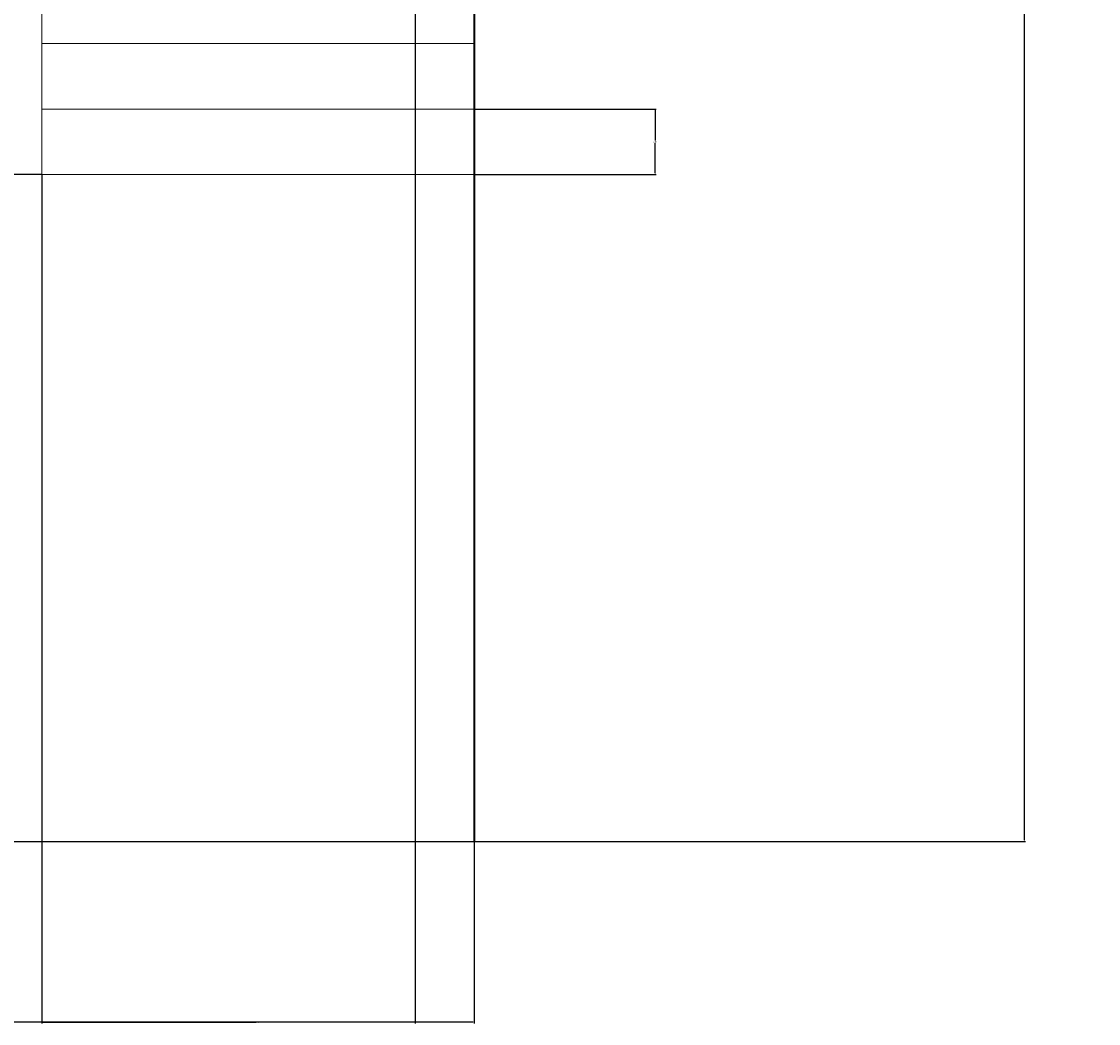
# Model space of a CAD drawing. Units: inches. Extents: x -4347 to -3836, y 955 to 1521.
# Tile 7 of 11: x -4001 to -3836, y 967 to 1120. Entities that reach past the tile are written whole.
import ezdxf

# ---------------------------------------------------------------- set-up
doc = ezdxf.new("R2010")
doc.units = ezdxf.units.IN
doc.header["$MEASUREMENT"] = 0
for name, color, linetype, lineweight in [('A-ANNO-DIMS', 2, 'Continuous', 18), ('A-FLOR', 7, 'Continuous', 25), ('A-FLOR-STRS', 7, 'Continuous', 18), ('A-WALL', 7, 'Continuous', 35)]:
    doc.layers.add(name, color=color, linetype=linetype, lineweight=lineweight)
doc.styles.get("Standard").update_dxf_attribs({"font": 'arial.ttf'})
doc.dimstyles.get("Standard").update_dxf_attribs({"dimtxt": 0.18, "dimasz": 0.18, "dimexe": 0.18, "dimexo": 0.0625, "dimgap": 0.09, "dimtad": 0, "dimtih": 1, "dimtoh": 1, "dimdec": 0, "dimzin": 0, "dimdsep": 46, "dimlunit": 3, "dimtxsty": 'Standard', "dimcen": 0.09, "dimadec": 0, "dimazin": 0, "dimtfac": 1, "dimtdec": 0, "dimtofl": 0, "dimtmove": 0, "dimatfit": 3, "dimfxl": 1, "dimtolj": 1, "dimtzin": 0, "dimarcsym": 0})

# ---------------------------------------------------------------- blocks, each defined once
blk = doc.blocks.new('*D2')
at = {"layer": 'A-ANNO-DIMS', "color": 0, "lineweight": -2, "transparency": 16777216}
for p, q in [((-3931.52, 1489.79), (-3847.29, 1489.79)), ((-3847.47, 1489.61), (-3847.47, 1245.44)), ((-3847.47, 994.97), (-3847.47, 1239.13)), ((-3931.52, 994.79), (-3847.29, 994.79))]:
    blk.add_line(p, q, dxfattribs=at)
at = {"layer": 'A-ANNO-DIMS', "color": 0, "transparency": 16777216}
for points in [[(-3847.5, 1489.61), (-3847.44, 1489.61), (-3847.47, 1489.79)], [(-3847.5, 994.97), (-3847.44, 994.97), (-3847.47, 994.79)]]:
    blk.add_solid(points, dxfattribs=at)
at = {"layer": 'Defpoints', "color": 0, "transparency": 16777216}
for p in [(-3931.58, 1489.79), (-3931.58, 994.79), (-3847.47, 994.79)]:
    blk.add_point(p, dxfattribs=at)
at = {"layer": 'A-ANNO-DIMS', "color": 0, "transparency": 16777216, "insert": (-3847.47, 1242.29), "char_height": 6, "attachment_point": 5}
blk.add_mtext('\\A1;41\'-3"', dxfattribs=at)
blk = doc.blocks.new('*D47')
at = {"layer": 'A-ANNO-DIMS', "color": 0, "lineweight": -2, "transparency": 16777216}
for p, q in [((-4120.58, 1288.73), (-4120.58, 966.96)), ((-3940.58, 1288.73), (-3940.58, 966.96)), ((-4120.4, 967.14), (-4030.97, 967.14)), ((-3940.76, 967.14), (-4030.19, 967.14))]:
    blk.add_line(p, q, dxfattribs=at)
at = {"layer": 'A-ANNO-DIMS', "color": 0, "transparency": 16777216}
for points in [[(-4120.4, 967.17), (-4120.4, 967.11), (-4120.58, 967.14)], [(-3940.76, 967.17), (-3940.76, 967.11), (-3940.58, 967.14)]]:
    blk.add_solid(points, dxfattribs=at)
at = {"layer": 'Defpoints', "color": 0, "transparency": 16777216}
for p in [(-4120.58, 1288.79), (-3940.58, 1288.79), (-3940.58, 967.14)]:
    blk.add_point(p, dxfattribs=at)
at = {"layer": 'A-ANNO-DIMS', "color": 0, "transparency": 16777216, "insert": (-4030.58, 967.14), "char_height": 0.18, "attachment_point": 5}
blk.add_mtext('\\A1;15\'-0"', dxfattribs=at)
blk = doc.blocks.new('*D52')
at = {"layer": 'A-ANNO-DIMS', "color": 0, "lineweight": -2, "transparency": 16777216}
for p, q in [((-3997.69, 1096.73), (-3997.69, 966.96)), ((-3931.58, 1096.73), (-3931.58, 966.96)), ((-3997.51, 967.14), (-3964.97, 967.14)), ((-3931.76, 967.14), (-3964.31, 967.14))]:
    blk.add_line(p, q, dxfattribs=at)
at = {"layer": 'A-ANNO-DIMS', "color": 0, "transparency": 16777216}
for points in [[(-3997.51, 967.17), (-3997.51, 967.11), (-3997.69, 967.14)], [(-3931.76, 967.17), (-3931.76, 967.11), (-3931.58, 967.14)]]:
    blk.add_solid(points, dxfattribs=at)
at = {"layer": 'Defpoints', "color": 0, "transparency": 16777216}
for p in [(-3997.69, 1096.79), (-3931.58, 1096.79), (-3931.58, 967.14)]:
    blk.add_point(p, dxfattribs=at)
at = {"layer": 'A-ANNO-DIMS', "color": 0, "transparency": 16777216, "insert": (-3964.64, 967.14), "char_height": 0.18, "attachment_point": 5}
blk.add_mtext('\\A1;5\'-6"', dxfattribs=at)
blk = doc.blocks.new('*D54')
at = {"layer": 'A-ANNO-DIMS', "color": 0, "lineweight": -2, "transparency": 16777216}
for p, q in [((-3997.76, 1126.79), (-4346.41, 1126.79)), ((-4346.23, 1126.61), (-4346.23, 1111.97)), ((-4346.23, 1096.97), (-4346.23, 1111.61)), ((-3997.76, 1096.79), (-4346.41, 1096.79))]:
    blk.add_line(p, q, dxfattribs=at)
at = {"layer": 'A-ANNO-DIMS', "color": 0, "transparency": 16777216}
for points in [[(-4346.26, 1126.61), (-4346.2, 1126.61), (-4346.23, 1126.79)], [(-4346.26, 1096.97), (-4346.2, 1096.97), (-4346.23, 1096.79)]]:
    blk.add_solid(points, dxfattribs=at)
at = {"layer": 'Defpoints', "color": 0, "transparency": 16777216}
for p in [(-4346.23, 1126.79), (-3997.69, 1126.79), (-3997.69, 1096.79)]:
    blk.add_point(p, dxfattribs=at)
at = {"layer": 'A-ANNO-DIMS', "color": 0, "transparency": 16777216, "insert": (-4346.23, 1111.79), "char_height": 0.18, "attachment_point": 5}
blk.add_mtext('\\A1;2\'-6"', dxfattribs=at)
blk = doc.blocks.new('*D55')
at = {"layer": 'A-ANNO-DIMS', "color": 0, "lineweight": -2, "transparency": 16777216}
for p, q in [((-3931.52, 1106.79), (-3903.75, 1106.79)), ((-3903.93, 1106.61), (-3903.93, 1101.97)), ((-3903.93, 1096.97), (-3903.93, 1101.61)), ((-3931.52, 1096.79), (-3903.75, 1096.79))]:
    blk.add_line(p, q, dxfattribs=at)
at = {"layer": 'A-ANNO-DIMS', "color": 0, "transparency": 16777216}
for points in [[(-3903.96, 1106.61), (-3903.9, 1106.61), (-3903.93, 1106.79)], [(-3903.96, 1096.97), (-3903.9, 1096.97), (-3903.93, 1096.79)]]:
    blk.add_solid(points, dxfattribs=at)
at = {"layer": 'Defpoints', "color": 0, "transparency": 16777216}
for p in [(-3931.58, 1106.79), (-3903.93, 1106.79), (-3931.58, 1096.79)]:
    blk.add_point(p, dxfattribs=at)
at = {"layer": 'A-ANNO-DIMS', "color": 0, "transparency": 16777216, "insert": (-3903.93, 1101.79), "char_height": 0.18, "attachment_point": 5}
blk.add_mtext('\\A1;0\'-10"', dxfattribs=at)

msp = doc.modelspace()

# ---------------------------------------------------------------- linework, layer by layer
at = {"layer": 'A-FLOR'}
msp.add_line((-4180.58, 994.79), (-3931.58, 994.79), dxfattribs=at)
at = {"layer": 'A-FLOR-STRS'}
for p, q in [((-3997.69, 1126.79), (-3997.69, 1116.79)), ((-3997.69, 1116.79), (-3997.69, 1106.79)), ((-3997.69, 1116.79), (-3931.58, 1116.79)), ((-3997.69, 1106.79), (-3997.69, 1096.79)), ((-3997.69, 1106.79), (-3931.58, 1106.79)), ((-3997.69, 1096.79), (-3931.58, 1096.79))]:
    msp.add_line(p, q, dxfattribs=at)
at = {"layer": 'A-WALL'}
msp.add_line((-3931.58, 1480.79), (-3931.58, 994.79), dxfattribs=at)

# ---------------------------------------------------------------- dimensions: what is measured, and where the dimension line sits
at = {"layer": 'A-ANNO-DIMS'}
for base, p1, p2, override, picture, middle in [((-3847.47, 994.79), (-3931.58, 1489.79), (-3931.58, 994.79), {"dimtxt": 6, "dimclrd": 0, "dimclre": 0, "dimclrt": 0}, '*D2', (-3847.47, 1242.29)), ((-4346.23, 1126.79), (-3997.69, 1096.79), (-3997.69, 1126.79), {"dimdec": 1, "dimlfac": 1, "dimrnd": 0, "dimzin": 1, "dimdsep": 46, "dimlunit": 4, "dimfrac": 2}, '*D54', (-4346.23, 1111.79)), ((-3903.93, 1106.79), (-3931.58, 1096.79), (-3931.58, 1106.79), {"dimdec": 1, "dimlfac": 1, "dimrnd": 0, "dimzin": 1, "dimdsep": 46, "dimlunit": 4, "dimfrac": 2}, '*D55', (-3903.93, 1101.79))]:
    dim = msp.add_linear_dim(base=base, p1=p1, p2=p2, angle=90, dimstyle='Standard', override=override, dxfattribs=at)
    dim.commit()
    dim.dimension.update_dxf_attribs({"geometry": picture, "text_midpoint": middle})
for base, p1, p2, picture, middle in [((-3940.58, 967.14), (-4120.58, 1288.79), (-3940.58, 1288.79), '*D47', (-4030.58, 967.14)), ((-3931.58, 967.14), (-3997.69, 1096.79), (-3931.58, 1096.79), '*D52', (-3964.64, 967.14))]:
    dim = msp.add_linear_dim(base=base, p1=p1, p2=p2, dimstyle='Standard', override={"dimdec": 1, "dimlfac": 1, "dimrnd": 0, "dimzin": 1, "dimdsep": 46, "dimlunit": 4, "dimfrac": 2}, dxfattribs=at)
    dim.commit()
    dim.dimension.update_dxf_attribs({"geometry": picture, "text_midpoint": middle})

doc.saveas('drawing.dxf')
